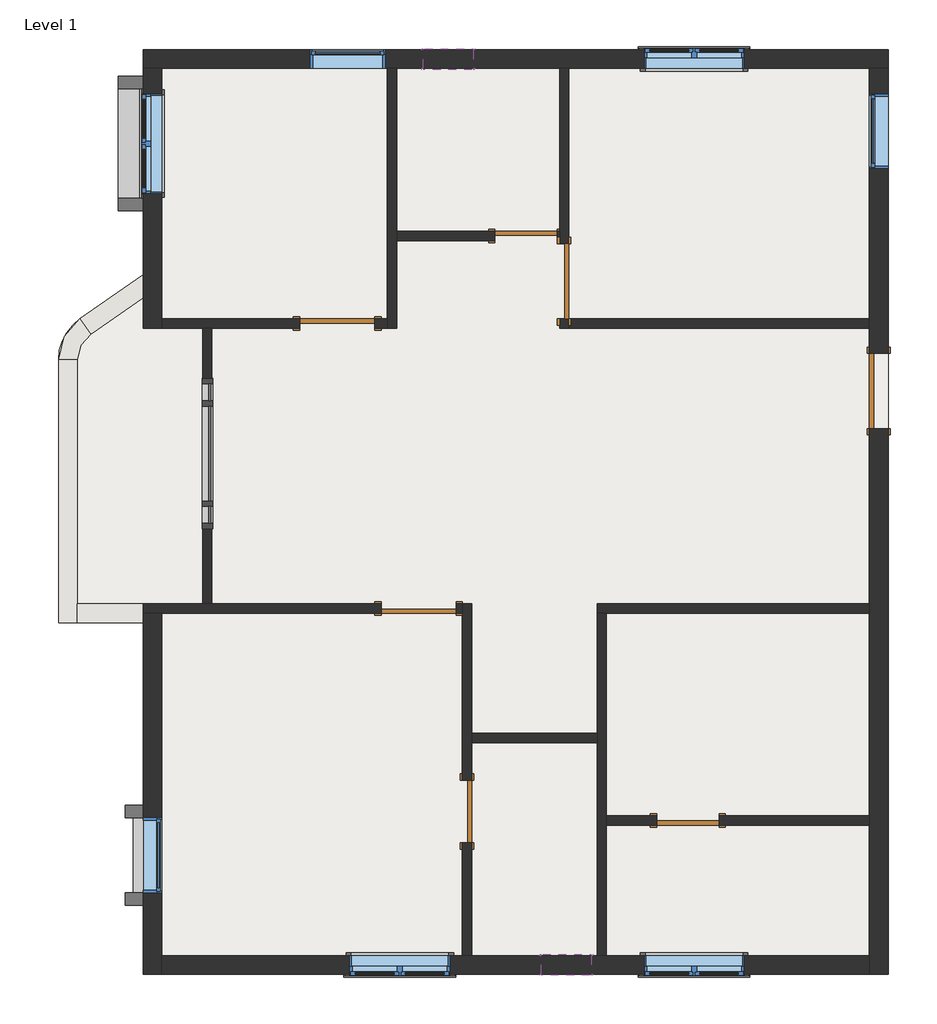
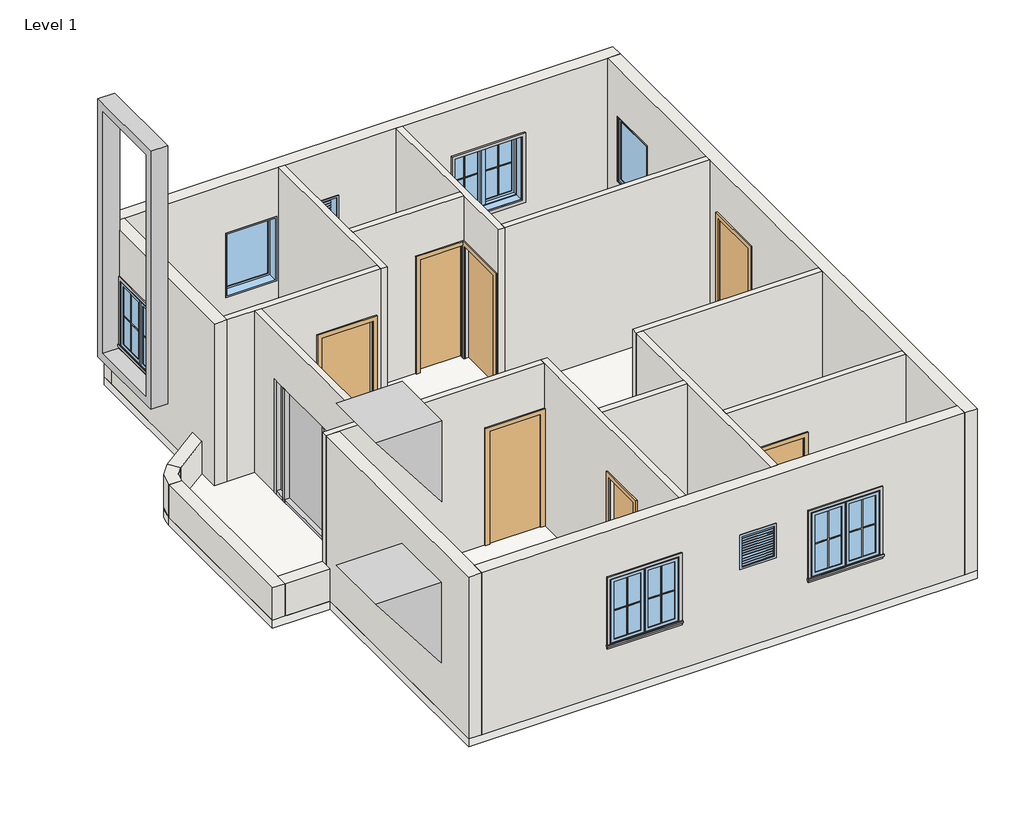
# One storey: 21 walls, 18 proxies, 9 windows, 7 doors, 7 members, 3 plates, 1 slab.
"""IFC4 building model written with IfcOpenShell, lengths in millimetres."""

from ifc_helpers import new_model, si_unit, point, frame, frame_2d, origin, origin_with_axes, place, context, project, spatial, polyline, circle_curve, trimmed, segment, composite_curve, outline, extrude, faceted_brep, transform, mapped, element, save
from components import generic_models_1_generic_models_1_7359c5b6, generic_models_2_generic_models_1_7ae53c19, muntin_pattern_2x2_muntin_pattern_2x2_4dfeb3f3, muntin_pattern_2x2_muntin_pattern_2x2_e852a7e4, trim_window_exterior_flat_with_sill_7cfdd449, trim_window_interior_flat_picture_frame_f1e0b15b, door_214872d5, door_78caadf7, door_e5f9f3c4, door_305aa2a5, door_0ca8825f, member_420b45ef, member_d7472725, member_7cbddb58, member_3374d9b6, system_panel_glazed_b82c55cd, system_panel_glazed_76d7ee11, window_c1f32544, window_af3140d2, window_f2d8fef0

model = new_model("IFC4")

# Units and contexts
model_context = context("Model", 3, world=origin())
ifc_project = project(units=[si_unit("LENGTHUNIT", "METRE", prefix="MILLI")], contexts=[model_context])

# Site, building, storey
site = spatial("IfcSite", under=ifc_project)
building = spatial("IfcBuilding", under=site)
storey = spatial("IfcBuildingStorey", under=building, Name="Level 1", Elevation=0.0)

# Proxies
placement = place(None, origin())
generic_models_1_generic_models_1_shape = generic_models_1_generic_models_1_7359c5b6(model_context)
element("IfcBuildingElementProxy", 1, Name="Generic Models 1 : Generic Models 1", ObjectType="Generic Models 1 : Generic Models 1", at=placement, inside=storey, context=model_context, shape_type="MappedRepresentation", body=[
    mapped(generic_models_1_generic_models_1_shape, transform((0.0, 0.0, 0.0), x_axis=(1.0, 0.0, 0.0), y_axis=(0.0, 1.0, 0.0), z_axis=(0.0, 0.0, 1.0))),
])
generic_models_2_generic_models_1_shape = generic_models_2_generic_models_1_7ae53c19(model_context)
element("IfcBuildingElementProxy", 2, Name="Generic Models 2 : Generic Models 1", ObjectType="Generic Models 2 : Generic Models 1", at=placement, inside=storey, context=model_context, shape_type="MappedRepresentation", body=[
    mapped(generic_models_2_generic_models_1_shape, transform((0.0, 0.0, 0.0), x_axis=(1.0, 0.0, 0.0), y_axis=(0.0, 1.0, 0.0), z_axis=(0.0, 0.0, 1.0))),
])
muntin_pattern_2x2_muntin_pattern_2x2_shape = muntin_pattern_2x2_muntin_pattern_2x2_4dfeb3f3(model_context)
element("IfcBuildingElementProxy", 3, Name="Muntin Pattern_2x2 : Muntin Pattern_2x2", ObjectType="Muntin Pattern_2x2 : Muntin Pattern_2x2", at=placement, inside=storey, context=model_context, shape_type="MappedRepresentation", body=[
    mapped(muntin_pattern_2x2_muntin_pattern_2x2_shape, transform((-15529.7981107, 3990.1340181, 984.25), x_axis=(0.0, 1.0, 0.0), y_axis=(-1.0, 0.0, 0.0), z_axis=(0.0, 0.0, 1.0))),
])
element("IfcBuildingElementProxy", 4, Name="Muntin Pattern_2x2 : Muntin Pattern_2x2", ObjectType="Muntin Pattern_2x2 : Muntin Pattern_2x2", at=placement, inside=storey, context=model_context, shape_type="MappedRepresentation", body=[
    mapped(muntin_pattern_2x2_muntin_pattern_2x2_shape, transform((-9136.9356107, 5426.8215181, 984.25), x_axis=(1.0, 0.0, 0.0), y_axis=(0.0, 1.0, 0.0), z_axis=(0.0, 0.0, 1.0))),
])
element("IfcBuildingElementProxy", 5, Name="Muntin Pattern_2x2 : Muntin Pattern_2x2", ObjectType="Muntin Pattern_2x2 : Muntin Pattern_2x2", at=placement, inside=storey, context=model_context, shape_type="MappedRepresentation", body=[
    mapped(muntin_pattern_2x2_muntin_pattern_2x2_shape, transform((-12111.9106107, -5806.3284819, 984.25), x_axis=(-1.0, 0.0, 0.0), y_axis=(0.0, -1.0, 0.0), z_axis=(0.0, 0.0, 1.0))),
])
element("IfcBuildingElementProxy", 6, Name="Muntin Pattern_2x2 : Muntin Pattern_2x2", ObjectType="Muntin Pattern_2x2 : Muntin Pattern_2x2", at=placement, inside=storey, context=model_context, shape_type="MappedRepresentation", body=[
    mapped(muntin_pattern_2x2_muntin_pattern_2x2_shape, transform((-8530.5106107, -5806.3284819, 984.25), x_axis=(-1.0, 0.0, 0.0), y_axis=(0.0, -1.0, 0.0), z_axis=(0.0, 0.0, 1.0))),
])
muntin_pattern_2x2_muntin_pattern_2x2_2_shape = muntin_pattern_2x2_muntin_pattern_2x2_e852a7e4(model_context)
element("IfcBuildingElementProxy", 7, Name="Muntin Pattern_2x2 : Muntin Pattern_2x2", ObjectType="Muntin Pattern_2x2 : Muntin Pattern_2x2", at=placement, inside=storey, context=model_context, shape_type="MappedRepresentation", body=[
    mapped(muntin_pattern_2x2_muntin_pattern_2x2_2_shape, transform((-15529.7981107, 4596.5590181, 984.25), x_axis=(0.0, -1.0, 0.0), y_axis=(1.0, 0.0, 0.0), z_axis=(0.0, 0.0, 1.0))),
])
element("IfcBuildingElementProxy", 8, Name="Muntin Pattern_2x2 : Muntin Pattern_2x2", ObjectType="Muntin Pattern_2x2 : Muntin Pattern_2x2", at=placement, inside=storey, context=model_context, shape_type="MappedRepresentation", body=[
    mapped(muntin_pattern_2x2_muntin_pattern_2x2_2_shape, transform((-8530.5106107, 5426.8215181, 984.25), x_axis=(-1.0, 0.0, 0.0), y_axis=(0.0, -1.0, 0.0), z_axis=(0.0, 0.0, 1.0))),
])
element("IfcBuildingElementProxy", 9, Name="Muntin Pattern_2x2 : Muntin Pattern_2x2", ObjectType="Muntin Pattern_2x2 : Muntin Pattern_2x2", at=placement, inside=storey, context=model_context, shape_type="MappedRepresentation", body=[
    mapped(muntin_pattern_2x2_muntin_pattern_2x2_2_shape, transform((-12718.3356107, -5806.3284819, 984.25), x_axis=(1.0, 0.0, 0.0), y_axis=(0.0, 1.0, 0.0), z_axis=(0.0, 0.0, 1.0))),
])
element("IfcBuildingElementProxy", 10, Name="Muntin Pattern_2x2 : Muntin Pattern_2x2", ObjectType="Muntin Pattern_2x2 : Muntin Pattern_2x2", at=placement, inside=storey, context=model_context, shape_type="MappedRepresentation", body=[
    mapped(muntin_pattern_2x2_muntin_pattern_2x2_2_shape, transform((-9136.9356107, -5806.3284819, 984.25), x_axis=(1.0, 0.0, 0.0), y_axis=(0.0, 1.0, 0.0), z_axis=(0.0, 0.0, 1.0))),
])
trim_window_exterior_flat_with_sill_shape = trim_window_exterior_flat_with_sill_7cfdd449(model_context)
element("IfcBuildingElementProxy", 11, Name="Trim-Window-Exterior-Flat : with Sill", ObjectType="Trim-Window-Exterior-Flat : with Sill", at=placement, inside=storey, context=model_context, shape_type="MappedRepresentation", body=[
    mapped(trim_window_exterior_flat_with_sill_shape, transform((-15539.3231107, 4293.3465181, 2133.6), x_axis=(0.0, -1.0, 0.0), y_axis=(0.0, 0.0, 1.0), z_axis=(-1.0, 0.0, 0.0))),
])
element("IfcBuildingElementProxy", 12, Name="Trim-Window-Exterior-Flat : with Sill", ObjectType="Trim-Window-Exterior-Flat : with Sill", at=placement, inside=storey, context=model_context, shape_type="MappedRepresentation", body=[
    mapped(trim_window_exterior_flat_with_sill_shape, transform((-8833.7231107, 5436.3465181, 2133.6), x_axis=(-1.0, 0.0, 0.0), y_axis=(0.0, 0.0, 1.0), z_axis=(0.0, 1.0, 0.0))),
])
element("IfcBuildingElementProxy", 13, Name="Trim-Window-Exterior-Flat : with Sill", ObjectType="Trim-Window-Exterior-Flat : with Sill", at=placement, inside=storey, context=model_context, shape_type="MappedRepresentation", body=[
    mapped(trim_window_exterior_flat_with_sill_shape, transform((-12415.1231107, -5815.8534819, 2133.6), x_axis=(1.0, 0.0, 0.0), y_axis=(0.0, 0.0, 1.0), z_axis=(0.0, -1.0, 0.0))),
])
element("IfcBuildingElementProxy", 14, Name="Trim-Window-Exterior-Flat : with Sill", ObjectType="Trim-Window-Exterior-Flat : with Sill", at=placement, inside=storey, context=model_context, shape_type="MappedRepresentation", body=[
    mapped(trim_window_exterior_flat_with_sill_shape, transform((-8833.7231107, -5815.8534819, 2133.6), x_axis=(1.0, 0.0, 0.0), y_axis=(0.0, 0.0, 1.0), z_axis=(0.0, -1.0, 0.0))),
])
trim_window_interior_flat_picture_frame_shape = trim_window_interior_flat_picture_frame_f1e0b15b(model_context)
element("IfcBuildingElementProxy", 15, Name="Trim-Window-Interior-Flat : Picture Frame", ObjectType="Trim-Window-Interior-Flat : Picture Frame", at=placement, inside=storey, context=model_context, shape_type="MappedRepresentation", body=[
    mapped(trim_window_interior_flat_picture_frame_shape, transform((-15310.7231107, 4293.3465181, 2133.6), x_axis=(0.0, 1.0, 0.0), y_axis=(0.0, 0.0, 1.0), z_axis=(1.0, 0.0, 0.0))),
])
element("IfcBuildingElementProxy", 16, Name="Trim-Window-Interior-Flat : Picture Frame", ObjectType="Trim-Window-Interior-Flat : Picture Frame", at=placement, inside=storey, context=model_context, shape_type="MappedRepresentation", body=[
    mapped(trim_window_interior_flat_picture_frame_shape, transform((-8833.7231107, 5207.7465181, 2133.6), x_axis=(1.0, 0.0, 0.0), y_axis=(0.0, 0.0, 1.0), z_axis=(0.0, -1.0, 0.0))),
])
element("IfcBuildingElementProxy", 17, Name="Trim-Window-Interior-Flat : Picture Frame", ObjectType="Trim-Window-Interior-Flat : Picture Frame", at=placement, inside=storey, context=model_context, shape_type="MappedRepresentation", body=[
    mapped(trim_window_interior_flat_picture_frame_shape, transform((-12415.1231107, -5587.2534819, 2133.6), x_axis=(-1.0, 0.0, 0.0), y_axis=(0.0, 0.0, 1.0), z_axis=(0.0, 1.0, 0.0))),
])
element("IfcBuildingElementProxy", 18, Name="Trim-Window-Interior-Flat : Picture Frame", ObjectType="Trim-Window-Interior-Flat : Picture Frame", at=placement, inside=storey, context=model_context, shape_type="MappedRepresentation", body=[
    mapped(trim_window_interior_flat_picture_frame_shape, transform((-8833.7231107, -5587.2534819, 2133.6), x_axis=(-1.0, 0.0, 0.0), y_axis=(0.0, 0.0, 1.0), z_axis=(0.0, 1.0, 0.0))),
])

# Doors
door_shape = door_214872d5(model_context)
element("IfcDoor", 19, ObjectType="Single-Flush : 2'6\" X 7'", at=placement, inside=storey, context=model_context, shape_type="MappedRepresentation", body=[
    mapped(door_shape, transform((-10878.4231107, 3169.3965181, 0.0), x_axis=(1.0, 0.0, 0.0), y_axis=(0.0, 1.0, 0.0), z_axis=(0.0, 0.0, 1.0))),
])
element("IfcDoor", 20, ObjectType="Single-Flush : 2'6\" X 7'", at=placement, inside=storey, context=model_context, shape_type="MappedRepresentation", body=[
    mapped(door_shape, transform((-8909.9231107, -3942.6034819, 0.0), x_axis=(-1.0, 0.0, 0.0), y_axis=(0.0, -1.0, 0.0), z_axis=(0.0, 0.0, 1.0))),
])
door_2_shape = door_78caadf7(model_context)
element("IfcDoor", 21, ObjectType="Single-Flush : 2'6\" X 7'", at=placement, inside=storey, context=model_context, shape_type="MappedRepresentation", body=[
    mapped(door_2_shape, transform((-11595.9731107, -3834.6534819, 0.0), x_axis=(0.0, 1.0, 0.0), y_axis=(-1.0, 0.0, 0.0), z_axis=(0.0, 0.0, 1.0))),
])
door_3_shape = door_e5f9f3c4(model_context)
element("IfcDoor", 22, ObjectType="Single-Flush : 36\" x 84\"", at=placement, inside=storey, context=model_context, shape_type="MappedRepresentation", body=[
    mapped(door_3_shape, transform((-13177.1231107, 2102.5965181, 0.0), x_axis=(1.0, 0.0, 0.0), y_axis=(0.0, 1.0, 0.0), z_axis=(0.0, 0.0, 1.0))),
])
element("IfcDoor", 23, ObjectType="Single-Flush : 36\" x 84\"", at=placement, inside=storey, context=model_context, shape_type="MappedRepresentation", body=[
    mapped(door_3_shape, transform((-10414.8731107, 2618.6439204, 0.0), x_axis=(0.0, -1.0, 0.0), y_axis=(1.0, 0.0, 0.0), z_axis=(0.0, 0.0, 1.0))),
])
door_4_shape = door_305aa2a5(model_context)
element("IfcDoor", 24, ObjectType="Single-Flush : 36\" x 84\"", at=placement, inside=storey, context=model_context, shape_type="MappedRepresentation", body=[
    mapped(door_4_shape, transform((-12186.5231107, -1364.5034819, 0.0), x_axis=(1.0, 0.0, 0.0), y_axis=(0.0, 1.0, 0.0), z_axis=(0.0, 0.0, 1.0))),
])
door_5_shape = door_0ca8825f(model_context)
element("IfcDoor", 25, ObjectType="Single-Flush : 36\" x 84\"", at=placement, inside=storey, context=model_context, shape_type="MappedRepresentation", body=[
    mapped(door_5_shape, transform((-6585.8231107, 1283.4465181, 0.0), x_axis=(0.0, 1.0, 0.0), y_axis=(-1.0, 0.0, 0.0), z_axis=(0.0, 0.0, 1.0))),
])

# Members
member_shape = member_420b45ef(model_context)
element("IfcMember", 26, ObjectType="Rectangular Mullion : 2.5\" x 5\" rectangular", at=placement, inside=storey, context=model_context, shape_type="MappedRepresentation", body=[
    mapped(member_shape, transform((-14758.2731107, 1372.3465181, 0.0), x_axis=(0.0, 0.0, -1.0), y_axis=(-1.0, 0.0, 0.0), z_axis=(0.0, 1.0, 0.0))),
])
element("IfcMember", 27, ObjectType="Rectangular Mullion : 2.5\" x 5\" rectangular", at=placement, inside=storey, context=model_context, shape_type="MappedRepresentation", body=[
    mapped(member_shape, transform((-14758.2731107, -119.9034819, 0.0), x_axis=(0.0, 0.0, -1.0), y_axis=(-1.0, 0.0, 0.0), z_axis=(0.0, 1.0, 0.0))),
])
member_2_shape = member_d7472725(model_context)
element("IfcMember", 28, ObjectType="Rectangular Mullion : 2.5\" x 5\" rectangular", at=placement, inside=storey, context=model_context, shape_type="MappedRepresentation", body=[
    mapped(member_2_shape, transform((-14758.2731107, 1099.2965181, 0.0), x_axis=(0.0, 0.0, -1.0), y_axis=(-1.0, 0.0, 0.0), z_axis=(0.0, 1.0, 0.0))),
])
member_3_shape = member_7cbddb58(model_context)
element("IfcMember", 29, ObjectType="Rectangular Mullion : 2.5\" x 5\" rectangular", at=placement, inside=storey, context=model_context, shape_type="MappedRepresentation", body=[
    mapped(member_3_shape, transform((-14758.2731107, 1131.0465181, 0.0), x_axis=(0.0, -1.0, 0.0), y_axis=(-1.0, 0.0, 0.0), z_axis=(0.0, 0.0, -1.0))),
])
element("IfcMember", 30, ObjectType="Rectangular Mullion : 2.5\" x 5\" rectangular", at=placement, inside=storey, context=model_context, shape_type="MappedRepresentation", body=[
    mapped(member_3_shape, transform((-14758.2731107, -88.1534819, 0.0), x_axis=(0.0, -1.0, 0.0), y_axis=(-1.0, 0.0, 0.0), z_axis=(0.0, 0.0, -1.0))),
])
member_4_shape = member_3374d9b6(model_context)
element("IfcMember", 31, ObjectType="Rectangular Mullion : 2.5\" x 5\" rectangular", at=placement, inside=storey, context=model_context, shape_type="MappedRepresentation", body=[
    mapped(member_4_shape, transform((-14758.2731107, 1435.8465181, 2133.6), x_axis=(0.0, 1.0, 0.0), y_axis=(-1.0, 0.0, 0.0), z_axis=(0.0, 0.0, 1.0))),
])
element("IfcMember", 32, ObjectType="Rectangular Mullion : 2.5\" x 5\" rectangular", at=placement, inside=storey, context=model_context, shape_type="MappedRepresentation", body=[
    mapped(member_4_shape, transform((-14758.2731107, -392.9534819, 0.0), x_axis=(0.0, -1.0, 0.0), y_axis=(-1.0, 0.0, 0.0), z_axis=(0.0, 0.0, -1.0))),
])

# Plates
system_panel_glazed_shape = system_panel_glazed_b82c55cd(model_context)
element("IfcPlate", 33, ObjectType="System Panel : Glazed", at=placement, inside=storey, context=model_context, shape_type="MappedRepresentation", body=[
    mapped(system_panel_glazed_shape, transform((-14758.2731107, 1267.5715181, 63.5), x_axis=(0.0, -1.0, 0.0), y_axis=(1.0, 0.0, 0.0), z_axis=(0.0, 0.0, 1.0))),
])
element("IfcPlate", 34, ObjectType="System Panel : Glazed", at=placement, inside=storey, context=model_context, shape_type="MappedRepresentation", body=[
    mapped(system_panel_glazed_shape, transform((-14758.2731107, -224.6784819, 63.5), x_axis=(0.0, -1.0, 0.0), y_axis=(1.0, 0.0, 0.0), z_axis=(0.0, 0.0, 1.0))),
])
system_panel_glazed_2_shape = system_panel_glazed_76d7ee11(model_context)
element("IfcPlate", 35, ObjectType="System Panel : Glazed", at=placement, inside=storey, context=model_context, shape_type="MappedRepresentation", body=[
    mapped(system_panel_glazed_2_shape, transform((-14758.2731107, 521.4465181, 63.5), x_axis=(0.0, -1.0, 0.0), y_axis=(1.0, 0.0, 0.0), z_axis=(0.0, 0.0, 1.0))),
])

# Slab
element("IfcSlab", 36, ObjectType="6\"", at=placement, inside=storey, context=model_context, shape_type="SweptSolid", body=[
    extrude(outline(composite_curve([segment(polyline([(-6471.5231107, 5436.3465181), (-6471.5231107, -5815.8534819), (-15539.3231107, -5815.8534819), (-15539.3231107, -1535.9534819), (-16568.0231107, -1535.9534819), (-16568.0231107, 1661.5585867)]), True, "CONTINUOUS"), segment(trimmed(circle_curve(frame_2d((-15958.4231107, 1661.5585867)), 609.6), [point((-16568.0231107, 1661.5585867))], [point((-16308.0753063, 2160.9136729))], False, "CARTESIAN"), True, "CONTINUOUS"), segment(polyline([(-16308.0753063, 2160.9136729), (-15539.3231107, 2699.1997553), (-15539.3231107, 5436.3465181), (-6471.5231107, 5436.3465181)]), True, "CONTINUOUS")], self_intersect=False)), frame((0.0, 0.0, -152.4), z_axis=(0.0, 0.0, 1.0), x_axis=(1.0, 0.0, 0.0)), (0.0, 0.0, 1.0), 152.4),
])

# Walls
element("IfcWall", 37, ObjectType="4.5\"", at=placement, inside=storey, context=model_context, shape_type="Brep", body=[
    faceted_brep([(-12567.5231107, 5207.7465181, 0.0), (-12567.5231107, 2159.7465181, 0.0), (-12567.5231107, 2045.4465181, 0.0), (-12567.5231107, 2045.4465181, 3048.0), (-12567.5231107, 2159.7465181, 3048.0), (-12567.5231107, 5207.7465181, 3048.0), (-12453.2231107, 5207.7465181, 0.0), (-12453.2231107, 5207.7465181, 3048.0), (-12453.2231107, 3226.5465181, 3048.0), (-12453.2231107, 3112.2465181, 3048.0), (-12453.2231107, 2045.4465181, 3048.0), (-12453.2231107, 2045.4465181, 0.0), (-12453.2231107, 3112.2465181, 0.0), (-12453.2231107, 3226.5465181, 0.0)], [[[0, 1, 2, 3, 4, 5]], [[6, 7, 8, 9, 10, 11, 12, 13]], [[2, 1, 0, 6, 13, 12, 11]], [[5, 4, 3, 10, 9, 8, 7]], [[0, 5, 7, 6]], [[3, 2, 11, 10]]]),
])
element("IfcWall", 38, ObjectType="4.5\"", at=placement, inside=storey, context=model_context, shape_type="Brep", body=[
    faceted_brep([(-12719.9231107, 2045.4465181, 2133.6), (-12719.9231107, 2045.4465181, 0.0), (-12567.5231107, 2045.4465181, 0.0), (-12567.5231107, 2045.4465181, 3048.0), (-14701.1231107, 2045.4465181, 3048.0), (-14815.4231107, 2045.4465181, 3048.0), (-15310.7231107, 2045.4465181, 3048.0), (-15310.7231107, 2045.4465181, 0.0), (-14815.4231107, 2045.4465181, 0.0), (-14701.1231107, 2045.4465181, 0.0), (-13634.3231107, 2045.4465181, 0.0), (-13634.3231107, 2045.4465181, 2133.6), (-12567.5231107, 2159.7465181, 0.0), (-12719.9231107, 2159.7465181, 0.0), (-12719.9231107, 2159.7465181, 2133.6), (-13634.3231107, 2159.7465181, 2133.6), (-13634.3231107, 2159.7465181, 0.0), (-15310.7231107, 2159.7465181, 0.0), (-15310.7231107, 2159.7465181, 3048.0), (-12567.5231107, 2159.7465181, 3048.0)], [[[0, 1, 2, 3, 4, 5, 6, 7, 8, 9, 10, 11]], [[12, 13, 14, 15, 16, 17, 18, 19]], [[2, 1, 13, 12]], [[10, 9, 8, 7, 17, 16]], [[6, 5, 4, 3, 19, 18]], [[3, 2, 12, 19]], [[7, 6, 18, 17]], [[14, 13, 1, 0]], [[15, 14, 0, 11]], [[16, 15, 11, 10]]]),
])
element("IfcWall", 39, ObjectType="4.5\"", at=placement, inside=storey, context=model_context, shape_type="Brep", body=[
    faceted_brep([(-10472.0231107, 2161.4439204, 2133.6), (-10472.0231107, 2161.4439204, 0.0), (-10472.0231107, 2045.4465181, 0.0), (-10472.0231107, 2045.4465181, 3048.0), (-10472.0231107, 3112.2465181, 3048.0), (-10472.0231107, 3226.5465181, 3048.0), (-10472.0231107, 5207.7465181, 3048.0), (-10472.0231107, 5207.7465181, 0.0), (-10472.0231107, 3226.5465181, 0.0), (-10472.0231107, 3112.2465181, 0.0), (-10472.0231107, 3075.8439204, 0.0), (-10472.0231107, 3075.8439204, 2133.6), (-10357.7231107, 2045.4465181, 0.0), (-10357.7231107, 2159.7465181, 0.0), (-10357.7231107, 2161.4439204, 0.0), (-10357.7231107, 2161.4439204, 2133.6), (-10357.7231107, 3075.8439204, 2133.6), (-10357.7231107, 3075.8439204, 0.0), (-10357.7231107, 5207.7465181, 0.0), (-10357.7231107, 5207.7465181, 3048.0), (-10357.7231107, 2159.7465181, 3048.0), (-10357.7231107, 2045.4465181, 3048.0)], [[[0, 1, 2, 3, 4, 5, 6, 7, 8, 9, 10, 11]], [[12, 13, 14, 15, 16, 17, 18, 19, 20, 21]], [[2, 1, 14, 13, 12]], [[10, 9, 8, 7, 18, 17]], [[6, 5, 4, 3, 21, 20, 19]], [[7, 6, 19, 18]], [[3, 2, 12, 21]], [[15, 14, 1, 0]], [[16, 15, 0, 11]], [[17, 16, 11, 10]]]),
])
element("IfcWall", 40, ObjectType="4.5\"", at=placement, inside=storey, context=model_context, shape_type="SweptSolid", body=[
    extrude(outline(polyline([(2133.6, -10497.4231107), (0.0, -10497.4231107), (0.0, -10472.0231107), (3048.0, -10472.0231107), (3048.0, -12453.2231107), (0.0, -12453.2231107), (0.0, -11259.4231107), (2133.6, -11259.4231107), (2133.6, -10497.4231107)])), frame((0.0, 3112.2465181, 0.0), z_axis=(0.0, 1.0, 0.0), x_axis=(0.0, 0.0, 1.0)), (0.0, 0.0, 1.0), 114.3),
])
element("IfcWall", 41, ObjectType="4.5\"", at=placement, inside=storey, context=model_context, shape_type="SweptSolid", body=[
    extrude(outline(polyline([(-10357.7231107, 2159.7465181), (-6700.1231107, 2159.7465181), (-6700.1231107, 2045.4465181), (-10357.7231107, 2045.4465181), (-10357.7231107, 2159.7465181)])), origin_with_axes(), (0.0, 0.0, 1.0), 3048.0),
])
element("IfcWall", 42, ObjectType="4.5\"", at=placement, inside=storey, context=model_context, shape_type="Brep", body=[
    faceted_brep([(-6700.1231107, -1307.3534819, 0.0), (-10014.8231107, -1307.3534819, 0.0), (-10014.8231107, -1307.3534819, 3048.0), (-6700.1231107, -1307.3534819, 3048.0), (-6700.1231107, -1421.6534819, 0.0), (-6700.1231107, -1421.6534819, 3048.0), (-9900.5231107, -1421.6534819, 3048.0), (-10014.8231107, -1421.6534819, 3048.0), (-10014.8231107, -1421.6534819, 0.0), (-9900.5231107, -1421.6534819, 0.0)], [[[0, 1, 2, 3]], [[4, 5, 6, 7, 8, 9]], [[1, 0, 4, 9, 8]], [[3, 2, 7, 6, 5]], [[0, 3, 5, 4]], [[2, 1, 8, 7]]]),
])
element("IfcWall", 43, ObjectType="4.5\"", at=placement, inside=storey, context=model_context, shape_type="SweptSolid", body=[
    extrude(outline(polyline([(0.0, -9900.5231107), (0.0, -9290.9231107), (2133.6, -9290.9231107), (2133.6, -8528.9231107), (0.0, -8528.9231107), (0.0, -6700.1231107), (3048.0, -6700.1231107), (3048.0, -9900.5231107), (0.0, -9900.5231107)])), frame((0.0, -3999.7534819, 0.0), z_axis=(0.0, 1.0, 0.0), x_axis=(0.0, 0.0, 1.0)), (0.0, 0.0, 1.0), 114.3),
])
element("IfcWall", 44, ObjectType="4.5\"", at=placement, inside=storey, context=model_context, shape_type="Brep", body=[
    faceted_brep([(-9900.5231107, -5587.2534819, 0.0), (-9900.5231107, -3999.7534819, 0.0), (-9900.5231107, -3885.4534819, 0.0), (-9900.5231107, -1421.6534819, 0.0), (-9900.5231107, -1421.6534819, 3048.0), (-9900.5231107, -3885.4534819, 3048.0), (-9900.5231107, -3999.7534819, 3048.0), (-9900.5231107, -5587.2534819, 3048.0), (-10014.8231107, -5587.2534819, 0.0), (-10014.8231107, -5587.2534819, 3048.0), (-10014.8231107, -2996.4534819, 3048.0), (-10014.8231107, -2882.1534819, 3048.0), (-10014.8231107, -1421.6534819, 3048.0), (-10014.8231107, -1421.6534819, 0.0), (-10014.8231107, -2882.1534819, 0.0), (-10014.8231107, -2996.4534819, 0.0)], [[[0, 1, 2, 3, 4, 5, 6, 7]], [[8, 9, 10, 11, 12, 13, 14, 15]], [[3, 2, 1, 0, 8, 15, 14, 13]], [[7, 6, 5, 4, 12, 11, 10, 9]], [[0, 7, 9, 8]], [[4, 3, 13, 12]]]),
])
element("IfcWall", 45, ObjectType="4.5\"", at=placement, inside=storey, context=model_context, shape_type="Brep", body=[
    faceted_brep([(-11538.8231107, -3453.6534819, 2133.6), (-11538.8231107, -3453.6534819, 0.0), (-11538.8231107, -2996.4534819, 0.0), (-11538.8231107, -2882.1534819, 0.0), (-11538.8231107, -1307.3534819, 0.0), (-11538.8231107, -1307.3534819, 3048.0), (-11538.8231107, -2882.1534819, 3048.0), (-11538.8231107, -2996.4534819, 3048.0), (-11538.8231107, -5587.2534819, 3048.0), (-11538.8231107, -5587.2534819, 0.0), (-11538.8231107, -4215.6534819, 0.0), (-11538.8231107, -4215.6534819, 2133.6), (-11653.1231107, -1307.3534819, 0.0), (-11653.1231107, -1421.6534819, 0.0), (-11653.1231107, -3453.6534819, 0.0), (-11653.1231107, -3453.6534819, 2133.6), (-11653.1231107, -4215.6534819, 2133.6), (-11653.1231107, -4215.6534819, 0.0), (-11653.1231107, -5587.2534819, 0.0), (-11653.1231107, -5587.2534819, 3048.0), (-11653.1231107, -1421.6534819, 3048.0), (-11653.1231107, -1307.3534819, 3048.0)], [[[0, 1, 2, 3, 4, 5, 6, 7, 8, 9, 10, 11]], [[12, 13, 14, 15, 16, 17, 18, 19, 20, 21]], [[10, 9, 18, 17]], [[4, 3, 2, 1, 14, 13, 12]], [[8, 7, 6, 5, 21, 20, 19]], [[9, 8, 19, 18]], [[5, 4, 12, 21]], [[15, 14, 1, 0]], [[16, 15, 0, 11]], [[17, 16, 11, 10]]]),
])
element("IfcWall", 46, ObjectType="4.5\"", at=placement, inside=storey, context=model_context, shape_type="SweptSolid", body=[
    extrude(outline(polyline([(-10014.8231107, -2996.4534819), (-11538.8231107, -2996.4534819), (-11538.8231107, -2882.1534819), (-10014.8231107, -2882.1534819), (-10014.8231107, -2996.4534819)])), origin_with_axes(), (0.0, 0.0, 1.0), 3048.0),
])
element("IfcWall", 47, ObjectType="4.5\"", at=placement, inside=storey, context=model_context, shape_type="Brep", body=[
    faceted_brep([(-11653.1231107, -1307.3534819, 0.0), (-11729.3231107, -1307.3534819, 0.0), (-11729.3231107, -1307.3534819, 2133.6), (-12643.7231107, -1307.3534819, 2133.6), (-12643.7231107, -1307.3534819, 0.0), (-14701.1231107, -1307.3534819, 0.0), (-14815.4231107, -1307.3534819, 0.0), (-15539.3231107, -1307.3534819, 0.0), (-15539.3231107, -1307.3534819, 609.6), (-15539.3231107, -1307.3534819, 3048.0), (-14815.4231107, -1307.3534819, 3048.0), (-14701.1231107, -1307.3534819, 3048.0), (-11653.1231107, -1307.3534819, 3048.0), (-11729.3231107, -1421.6534819, 2133.6), (-11729.3231107, -1421.6534819, 0.0), (-11653.1231107, -1421.6534819, 0.0), (-11653.1231107, -1421.6534819, 3048.0), (-15310.7231107, -1421.6534819, 3048.0), (-15539.3231107, -1421.6534819, 3048.0), (-15539.3231107, -1421.6534819, 0.0), (-15310.7231107, -1421.6534819, 0.0), (-12643.7231107, -1421.6534819, 0.0), (-12643.7231107, -1421.6534819, 2133.6)], [[[0, 1, 2, 3, 4, 5, 6, 7, 8, 9, 10, 11, 12]], [[13, 14, 15, 16, 17, 18, 19, 20, 21, 22]], [[15, 14, 1, 0]], [[21, 20, 19, 7, 6, 5, 4]], [[12, 11, 10, 9, 18, 17, 16]], [[0, 12, 16, 15]], [[2, 1, 14, 13]], [[3, 2, 13, 22]], [[4, 3, 22, 21]], [[7, 19, 18, 9, 8]]]),
])
element("IfcWall", 48, ObjectType="4.5\"", at=placement, inside=storey, context=model_context, shape_type="SweptSolid", body=[
    extrude(outline(polyline([(-1307.3534819, 3048.0), (2045.4465181, 3048.0), (2045.4465181, 0.0), (1435.8465181, 0.0), (1435.8465181, 2133.6), (-392.9534819, 2133.6), (-392.9534819, 0.0), (-1307.3534819, 0.0), (-1307.3534819, 3048.0)])), frame((-14815.4231107, 0.0, 0.0), z_axis=(1.0, 0.0, 0.0), x_axis=(0.0, 1.0, 0.0)), (0.0, 0.0, 1.0), 114.3),
])
element("IfcWall", 49, ObjectType="9\"", at=placement, inside=storey, context=model_context, shape_type="Brep", body=[
    faceted_brep([(-15539.3231107, 5207.7465181, 0.0), (-15310.7231107, 5207.7465181, 0.0), (-12567.5231107, 5207.7465181, 0.0), (-12453.2231107, 5207.7465181, 0.0), (-10472.0231107, 5207.7465181, 0.0), (-10357.7231107, 5207.7465181, 0.0), (-6700.1231107, 5207.7465181, 0.0), (-6471.5231107, 5207.7465181, 0.0), (-6471.5231107, 5207.7465181, 3048.0), (-6700.1231107, 5207.7465181, 3048.0), (-10357.7231107, 5207.7465181, 3048.0), (-10472.0231107, 5207.7465181, 3048.0), (-12453.2231107, 5207.7465181, 3048.0), (-12567.5231107, 5207.7465181, 3048.0), (-15310.7231107, 5207.7465181, 3048.0), (-15539.3231107, 5207.7465181, 3048.0), (-12129.3731107, 5207.7465181, 2133.6), (-11519.7731107, 5207.7465181, 2133.6), (-11519.7731107, 5207.7465181, 1524.0), (-12129.3731107, 5207.7465181, 1524.0), (-8224.1231107, 5207.7465181, 2133.6), (-8224.1231107, 5207.7465181, 914.4), (-9443.3231107, 5207.7465181, 914.4), (-9443.3231107, 5207.7465181, 2133.6), (-12592.9231107, 5207.7465181, 2133.6), (-12592.9231107, 5207.7465181, 914.4), (-13507.3231107, 5207.7465181, 914.4), (-13507.3231107, 5207.7465181, 2133.6), (-15539.3231107, 5436.3465181, 0.0), (-15539.3231107, 5436.3465181, 3048.0), (-6471.5231107, 5436.3465181, 3048.0), (-6471.5231107, 5436.3465181, 0.0), (-12129.3731107, 5436.3465181, 2133.6), (-12129.3731107, 5436.3465181, 1524.0), (-11519.7731107, 5436.3465181, 1524.0), (-11519.7731107, 5436.3465181, 2133.6), (-8224.1231107, 5436.3465181, 2133.6), (-9443.3231107, 5436.3465181, 2133.6), (-9443.3231107, 5436.3465181, 914.4), (-8224.1231107, 5436.3465181, 914.4), (-12592.9231107, 5436.3465181, 2133.6), (-13507.3231107, 5436.3465181, 2133.6), (-13507.3231107, 5436.3465181, 914.4), (-12592.9231107, 5436.3465181, 914.4)], [[[0, 1, 2, 3, 4, 5, 6, 7, 8, 9, 10, 11, 12, 13, 14, 15], [16, 17, 18, 19], [20, 21, 22, 23], [24, 25, 26, 27]], [[28, 29, 30, 31], [32, 33, 34, 35], [36, 37, 38, 39], [40, 41, 42, 43]], [[7, 6, 5, 4, 3, 2, 1, 0, 28, 31]], [[15, 14, 13, 12, 11, 10, 9, 8, 30, 29]], [[0, 15, 29, 28]], [[8, 7, 31, 30]], [[33, 32, 16, 19]], [[34, 33, 19, 18]], [[35, 34, 18, 17]], [[32, 35, 17, 16]], [[21, 20, 36, 39]], [[22, 21, 39, 38]], [[23, 22, 38, 37]], [[20, 23, 37, 36]], [[25, 24, 40, 43]], [[26, 25, 43, 42]], [[27, 26, 42, 41]], [[24, 27, 41, 40]]]),
])
element("IfcWall", 50, ObjectType="9\"", at=placement, inside=storey, context=model_context, shape_type="Brep", body=[
    faceted_brep([(-15539.3231107, 5207.7465181, 0.0), (-15539.3231107, 2699.1997553, 0.0), (-15539.3231107, 2420.1306843, 0.0), (-15539.3231107, 2045.4465181, 0.0), (-15539.3231107, 2045.4465181, 3048.0), (-15539.3231107, 5207.7465181, 3048.0), (-15539.3231107, 4902.9465181, 2133.6), (-15539.3231107, 3683.7465181, 2133.6), (-15539.3231107, 3683.7465181, 914.4), (-15539.3231107, 4902.9465181, 914.4), (-15310.7231107, 5207.7465181, 0.0), (-15310.7231107, 5207.7465181, 3048.0), (-15310.7231107, 2159.7465181, 3048.0), (-15310.7231107, 2045.4465181, 3048.0), (-15310.7231107, 2045.4465181, 0.0), (-15310.7231107, 2159.7465181, 0.0), (-15310.7231107, 4902.9465181, 2133.6), (-15310.7231107, 4902.9465181, 914.4), (-15310.7231107, 3683.7465181, 914.4), (-15310.7231107, 3683.7465181, 2133.6)], [[[0, 1, 2, 3, 4, 5], [6, 7, 8, 9]], [[10, 11, 12, 13, 14, 15], [16, 17, 18, 19]], [[3, 2, 1, 0, 10, 15, 14]], [[5, 4, 13, 12, 11]], [[0, 5, 11, 10]], [[4, 3, 14, 13]], [[17, 16, 6, 9]], [[18, 17, 9, 8]], [[19, 18, 8, 7]], [[16, 19, 7, 6]]]),
])
element("IfcWall", 51, ObjectType="9\"", at=placement, inside=storey, context=model_context, shape_type="Brep", body=[
    faceted_brep([(-6700.1231107, 5207.7465181, 0.0), (-6700.1231107, 2159.7465181, 0.0), (-6700.1231107, 2045.4465181, 0.0), (-6700.1231107, 1740.6465181, 0.0), (-6700.1231107, 1740.6465181, 2133.6), (-6700.1231107, 826.2465181, 2133.6), (-6700.1231107, 826.2465181, 0.0), (-6700.1231107, -1307.3534819, 0.0), (-6700.1231107, -1421.6534819, 0.0), (-6700.1231107, -3885.4534819, 0.0), (-6700.1231107, -3999.7534819, 0.0), (-6700.1231107, -5587.2534819, 0.0), (-6700.1231107, -5815.8534819, 0.0), (-6700.1231107, -5815.8534819, 3048.0), (-6700.1231107, -5587.2534819, 3048.0), (-6700.1231107, -3999.7534819, 3048.0), (-6700.1231107, -3885.4534819, 3048.0), (-6700.1231107, -1421.6534819, 3048.0), (-6700.1231107, -1307.3534819, 3048.0), (-6700.1231107, 2045.4465181, 3048.0), (-6700.1231107, 2159.7465181, 3048.0), (-6700.1231107, 5207.7465181, 3048.0), (-6700.1231107, 4902.9465181, 2133.6), (-6700.1231107, 3988.5465181, 2133.6), (-6700.1231107, 3988.5465181, 914.4), (-6700.1231107, 4902.9465181, 914.4), (-6471.5231107, 1740.6465181, 2133.6), (-6471.5231107, 1740.6465181, 0.0), (-6471.5231107, 5207.7465181, 0.0), (-6471.5231107, 5207.7465181, 3048.0), (-6471.5231107, -5815.8534819, 3048.0), (-6471.5231107, -5815.8534819, 0.0), (-6471.5231107, 826.2465181, 0.0), (-6471.5231107, 826.2465181, 2133.6), (-6471.5231107, 4902.9465181, 2133.6), (-6471.5231107, 4902.9465181, 914.4), (-6471.5231107, 3988.5465181, 914.4), (-6471.5231107, 3988.5465181, 2133.6)], [[[0, 1, 2, 3, 4, 5, 6, 7, 8, 9, 10, 11, 12, 13, 14, 15, 16, 17, 18, 19, 20, 21], [22, 23, 24, 25]], [[26, 27, 28, 29, 30, 31, 32, 33], [34, 35, 36, 37]], [[32, 31, 12, 11, 10, 9, 8, 7, 6]], [[28, 27, 3, 2, 1, 0]], [[21, 20, 19, 18, 17, 16, 15, 14, 13, 30, 29]], [[0, 21, 29, 28]], [[13, 12, 31, 30]], [[35, 34, 22, 25]], [[36, 35, 25, 24]], [[37, 36, 24, 23]], [[34, 37, 23, 22]], [[4, 3, 27, 26]], [[5, 4, 26, 33]], [[6, 5, 33, 32]]]),
])
element("IfcWall", 52, ObjectType="9\"", at=placement, inside=storey, context=model_context, shape_type="Brep", body=[
    faceted_brep([(-15310.7231107, -5815.8534819, 0.0), (-6700.1231107, -5815.8534819, 0.0), (-6700.1231107, -5815.8534819, 3048.0), (-15310.7231107, -5815.8534819, 3048.0), (-10084.6731107, -5815.8534819, 2133.6), (-10084.6731107, -5815.8534819, 1524.0), (-10694.2731107, -5815.8534819, 1524.0), (-10694.2731107, -5815.8534819, 2133.6), (-13024.7231107, -5815.8534819, 2133.6), (-11805.5231107, -5815.8534819, 2133.6), (-11805.5231107, -5815.8534819, 914.4), (-13024.7231107, -5815.8534819, 914.4), (-9443.3231107, -5815.8534819, 2133.6), (-8224.1231107, -5815.8534819, 2133.6), (-8224.1231107, -5815.8534819, 914.4), (-9443.3231107, -5815.8534819, 914.4), (-15310.7231107, -5587.2534819, 0.0), (-15310.7231107, -5587.2534819, 3048.0), (-11653.1231107, -5587.2534819, 3048.0), (-11538.8231107, -5587.2534819, 3048.0), (-10014.8231107, -5587.2534819, 3048.0), (-9900.5231107, -5587.2534819, 3048.0), (-6700.1231107, -5587.2534819, 3048.0), (-6700.1231107, -5587.2534819, 0.0), (-9900.5231107, -5587.2534819, 0.0), (-10014.8231107, -5587.2534819, 0.0), (-11538.8231107, -5587.2534819, 0.0), (-11653.1231107, -5587.2534819, 0.0), (-10084.6731107, -5587.2534819, 2133.6), (-10694.2731107, -5587.2534819, 2133.6), (-10694.2731107, -5587.2534819, 1524.0), (-10084.6731107, -5587.2534819, 1524.0), (-13024.7231107, -5587.2534819, 2133.6), (-13024.7231107, -5587.2534819, 914.4), (-11805.5231107, -5587.2534819, 914.4), (-11805.5231107, -5587.2534819, 2133.6), (-9443.3231107, -5587.2534819, 2133.6), (-9443.3231107, -5587.2534819, 914.4), (-8224.1231107, -5587.2534819, 914.4), (-8224.1231107, -5587.2534819, 2133.6)], [[[0, 1, 2, 3], [4, 5, 6, 7], [8, 9, 10, 11], [12, 13, 14, 15]], [[16, 17, 18, 19, 20, 21, 22, 23, 24, 25, 26, 27], [28, 29, 30, 31], [32, 33, 34, 35], [36, 37, 38, 39]], [[1, 0, 16, 27, 26, 25, 24, 23]], [[3, 2, 22, 21, 20, 19, 18, 17]], [[0, 3, 17, 16]], [[2, 1, 23, 22]], [[5, 4, 28, 31]], [[6, 5, 31, 30]], [[7, 6, 30, 29]], [[4, 7, 29, 28]], [[33, 32, 8, 11]], [[34, 33, 11, 10]], [[35, 34, 10, 9]], [[32, 35, 9, 8]], [[37, 36, 12, 15]], [[38, 37, 15, 14]], [[39, 38, 14, 13]], [[36, 39, 13, 12]]]),
])
element("IfcWall", 53, ObjectType="9\"", at=placement, inside=storey, context=model_context, shape_type="Brep", body=[
    faceted_brep([(-15539.3231107, -1421.6534819, 3048.0), (-15539.3231107, -1421.6534819, 0.0), (-15539.3231107, -1535.9534819, 0.0), (-15539.3231107, -5815.8534819, 0.0), (-15539.3231107, -5815.8534819, 3048.0), (-15539.3231107, -4825.2534819, 2133.6), (-15539.3231107, -4825.2534819, 914.4), (-15539.3231107, -3910.8534819, 914.4), (-15539.3231107, -3910.8534819, 2133.6), (-15310.7231107, -1421.6534819, 0.0), (-15310.7231107, -1421.6534819, 3048.0), (-15310.7231107, -5587.2534819, 3048.0), (-15310.7231107, -5815.8534819, 3048.0), (-15310.7231107, -5815.8534819, 0.0), (-15310.7231107, -5587.2534819, 0.0), (-15310.7231107, -4825.2534819, 2133.6), (-15310.7231107, -3910.8534819, 2133.6), (-15310.7231107, -3910.8534819, 914.4), (-15310.7231107, -4825.2534819, 914.4)], [[[0, 1, 2, 3, 4], [5, 6, 7, 8]], [[9, 10, 11, 12, 13, 14], [15, 16, 17, 18]], [[3, 2, 1, 9, 14, 13]], [[0, 4, 12, 11, 10]], [[4, 3, 13, 12]], [[0, 10, 9, 1]], [[6, 5, 15, 18]], [[7, 6, 18, 17]], [[8, 7, 17, 16]], [[5, 8, 16, 15]]]),
])
element("IfcWall", 54, ObjectType="9\"", at=placement, inside=storey, context=model_context, shape_type="Brep", body=[
    faceted_brep([(-16339.4231107, -1535.9534819, 0.0), (-16339.4231107, -1307.3534819, 0.0), (-16339.4231107, 1661.5585867, 0.0), (-16339.4231107, 1661.5585867, 609.6), (-16339.4231107, -1307.3534819, 609.6), (-16339.4231107, -1535.9534819, 609.6), (-16568.0231107, -1535.9534819, 0.0), (-16568.0231107, -1535.9534819, 609.6), (-16568.0231107, 1661.5585867, 609.6), (-16568.0231107, 1661.5585867, 0.0)], [[[0, 1, 2, 3, 4, 5]], [[6, 7, 8, 9]], [[2, 1, 0, 6, 9]], [[3, 2, 9, 8]], [[5, 4, 3, 8, 7]], [[0, 5, 7, 6]]]),
])
element("IfcWall", 55, ObjectType="9\"", at=placement, inside=storey, context=model_context, shape_type="Brep", body=[
    faceted_brep([(-15539.3231107, -1307.3534819, 0.0), (-16339.4231107, -1307.3534819, 0.0), (-16339.4231107, -1307.3534819, 609.6), (-15539.3231107, -1307.3534819, 609.6), (-15539.3231107, -1535.9534819, 0.0), (-15539.3231107, -1535.9534819, 609.6), (-16339.4231107, -1535.9534819, 609.6), (-16339.4231107, -1535.9534819, 0.0), (-15539.3231107, -1421.6534819, 0.0)], [[[0, 1, 2, 3]], [[4, 5, 6, 7]], [[1, 0, 8, 4, 7]], [[3, 2, 6, 5]], [[0, 3, 5, 4, 8]], [[2, 1, 7, 6]]]),
])
element("IfcWall", 56, ObjectType="9\"", at=placement, inside=storey, context=model_context, shape_type="SweptSolid", body=[
    extrude(outline(polyline([(-15539.3231107, 2420.1306843), (-16176.9557329, 1973.6555156), (-16308.0753063, 2160.9136729), (-15539.3231107, 2699.1997553), (-15539.3231107, 2420.1306843)])), origin_with_axes(), (0.0, 0.0, 1.0), 609.6),
])
element("IfcWall", 57, ObjectType="9\"", at=placement, inside=storey, context=model_context, shape_type="SweptSolid", body=[
    extrude(outline(composite_curve([segment(polyline([(-16308.0753063, 2160.9136729), (-16176.9557329, 1973.6555156)]), True, "CONTINUOUS"), segment(trimmed(circle_curve(frame_2d((-15958.4231107, 1661.5585867)), 381.0), [point((-16176.9557329, 1973.6555156))], [point((-16339.4231107, 1661.5585867))], True, "CARTESIAN"), True, "CONTINUOUS"), segment(polyline([(-16339.4231107, 1661.5585867), (-16568.0231107, 1661.5585867)]), True, "CONTINUOUS"), segment(trimmed(circle_curve(frame_2d((-15958.4231107, 1661.5585867)), 609.6), [point((-16568.0231107, 1661.5585867))], [point((-16308.0753063, 2160.9136729))], False, "CARTESIAN"), True, "CONTINUOUS")], self_intersect=False)), origin_with_axes(), (0.0, 0.0, 1.0), 609.6),
])

# Windows
window_shape = window_c1f32544(model_context)
element("IfcWindow", 58, ObjectType="Fixed : 36\" x 48\"", at=placement, inside=storey, context=model_context, shape_type="MappedRepresentation", body=[
    mapped(window_shape, transform((-13012.0231107, 5322.0465181, 0.0), x_axis=(1.0, 0.0, 0.0), y_axis=(0.0, 1.0, 0.0), z_axis=(0.0, 0.0, 1.0))),
])
element("IfcWindow", 59, ObjectType="Fixed : 36\" x 48\"", at=placement, inside=storey, context=model_context, shape_type="MappedRepresentation", body=[
    mapped(window_shape, transform((-6585.8231107, 4483.8465181, 0.0), x_axis=(0.0, 1.0, 0.0), y_axis=(-1.0, 0.0, 0.0), z_axis=(0.0, 0.0, 1.0))),
])
element("IfcWindow", 60, ObjectType="Fixed : 36\" x 48\"", at=placement, inside=storey, context=model_context, shape_type="MappedRepresentation", body=[
    mapped(window_shape, transform((-15425.0231107, -4406.1534819, 0.0), x_axis=(0.0, -1.0, 0.0), y_axis=(1.0, 0.0, 0.0), z_axis=(0.0, 0.0, 1.0))),
])
window_2_shape = window_af3140d2(model_context)
element("IfcWindow", 61, ObjectType="Window-Casement-Double : 48\" x 48\"", at=placement, inside=storey, context=model_context, shape_type="MappedRepresentation", body=[
    mapped(window_2_shape, transform((-15425.0231107, 4293.3465181, 0.0), x_axis=(0.0, 1.0, 0.0), y_axis=(-1.0, 0.0, 0.0), z_axis=(0.0, 0.0, 1.0))),
])
element("IfcWindow", 62, ObjectType="Window-Casement-Double : 48\" x 48\"", at=placement, inside=storey, context=model_context, shape_type="MappedRepresentation", body=[
    mapped(window_2_shape, transform((-8833.7231107, 5322.0465181, 0.0), x_axis=(1.0, 0.0, 0.0), y_axis=(0.0, 1.0, 0.0), z_axis=(0.0, 0.0, 1.0))),
])
element("IfcWindow", 63, ObjectType="Window-Casement-Double : 48\" x 48\"", at=placement, inside=storey, context=model_context, shape_type="MappedRepresentation", body=[
    mapped(window_2_shape, transform((-12415.1231107, -5701.5534819, 0.0), x_axis=(-1.0, 0.0, 0.0), y_axis=(0.0, -1.0, 0.0), z_axis=(0.0, 0.0, 1.0))),
])
element("IfcWindow", 64, ObjectType="Window-Casement-Double : 48\" x 48\"", at=placement, inside=storey, context=model_context, shape_type="MappedRepresentation", body=[
    mapped(window_2_shape, transform((-8833.7231107, -5701.5534819, 0.0), x_axis=(-1.0, 0.0, 0.0), y_axis=(0.0, -1.0, 0.0), z_axis=(0.0, 0.0, 1.0))),
])
window_3_shape = window_f2d8fef0(model_context)
element("IfcWindow", 65, ObjectType="Window-Louvers : 24\" x 24\"", at=placement, inside=storey, context=model_context, shape_type="MappedRepresentation", body=[
    mapped(window_3_shape, transform((-11824.5731107, 5328.3965181, 609.6), x_axis=(1.0, 0.0, 0.0), y_axis=(0.0, 1.0, 0.0), z_axis=(0.0, 0.0, 1.0))),
])
element("IfcWindow", 66, ObjectType="Window-Louvers : 24\" x 24\"", at=placement, inside=storey, context=model_context, shape_type="MappedRepresentation", body=[
    mapped(window_3_shape, transform((-10389.4731107, -5707.9034819, 609.6), x_axis=(-1.0, 0.0, 0.0), y_axis=(0.0, -1.0, 0.0), z_axis=(0.0, 0.0, 1.0))),
])

save(model, "model.ifc")

# Revit data of these elements
# Type "Muntin Pattern_2x2 : Muntin Pattern_2x2"
#   Width [instance default] = 4' - 0"
#   Thickness = 0' - 0 1/2"
#   Height [instance default] = 4' - 0"
#   Distance = 0' - 0 3/4"
#   Interior Material [instance default] = none
#   Exterior Material [instance default] = none
#   Default Elevation = 0
# Type "Trim-Window-Exterior-Flat : with Sill"
#   Trim Width = 0' - 2 1/4"
#   Trim Thickness_Picture Frame = 0' - 1 1/4"
#   Trim Thickness_with Sill = 0' - 0 3/4"
#   Sill Thickness = 0' - 1 1/4"
#   Opening Width [instance default] = 2' - 0"
#   Opening Height [instance default] = 3' - 0"
#   Default Elevation = 4' - 0"
#   Sill = yes
#   Picture Frame = no
#   Trim Material [instance default] = none
# Type "Trim-Window-Interior-Flat : Picture Frame"
#   Trim Thickness_Picture Frame = 0' - 1 1/4"
#   Trim Width = 0' - 2 1/4"
#   Trim Thickness_with Sill = 0' - 0 3/4"
#   Sill Thickness = 0' - 1 1/4"
#   Opening Width [instance default] = 2' - 0"
#   Opening Height [instance default] = 3' - 0"
#   Default Elevation = 4' - 0"
#   Sill = no
#   Picture Frame = yes
#   Trim Material [instance default] = none
# Type "Single-Flush : 2'6\" X 7'"
#   Type Mark = "8"
#   Construction Type Id = "MDOOR"
#   Assembly Code = "C1020"
#   Analytic Construction = "Metal"
#   Thickness = 0' - 2"
#   Heat Transfer Coefficient (U) = 0.651978 BTU/(h·ft²·°F)
#   Height = 7' - 0"
#   Trim Projection Ext = 0' - 1"
#   Trim Projection Int = 0' - 1"
#   Trim Width = 0' - 3"
#   Width = 2' - 6"
#   Define Thermal Properties by = 1
#   Door Material = Door - Panel
#   Frame Material = Door - Frame
#   Visual Light Transmittance = 0
#   Solar Heat Gain Coefficient = 0
#   Function = (empty or 0)
#   Wall Closure = (empty or 0)
# Type "Single-Flush : 36\" x 84\""
#   Type Mark = "1"
#   Construction Type Id = "MDOOR"
#   Assembly Code = "C1020"
#   Analytic Construction = "Metal"
#   Thickness = 0' - 2"
#   Heat Transfer Coefficient (U) = 0.651978 BTU/(h·ft²·°F)
#   Height = 7' - 0"
#   Trim Projection Ext = 0' - 1"
#   Trim Projection Int = 0' - 1"
#   Trim Width = 0' - 3"
#   Width = 3' - 0"
#   Define Thermal Properties by = 1
#   Define Thermal Properties by = 1
#   Door Material = Door - Panel
#   Frame Material = Door - Frame
#   Visual Light Transmittance = 0
#   Solar Heat Gain Coefficient = 0
#   Function = (empty or 0)
#   Wall Closure = (empty or 0)
# Type "Rectangular Mullion : 2.5\" x 5\" rectangular"
#   built-in parameter 1007304 = 0.416667 (stored number, unit not read)
#   built-in parameter 1007301 = 0.104167 (stored number, unit not read)
#   built-in parameter 1007300 = 0.104167 (stored number, unit not read)
# Type "System Panel : Glazed"
#   Construction Type Id = "GSP4R"
#   Analytic Construction = "1/8 in Pilkington single glazing"
#   Visual Light Transmittance = 0.9
#   Solar Heat Gain Coefficient = 0.86
#   Heat Transfer Coefficient (U) = 1.18115 BTU/(h·ft²·°F)
#   Define Thermal Properties by = 1
# Type "6\""
#   Assembly Code = "B1010"
#   Function = 0
#   Layers, outside or top first: 0' - 6" no material (function 1)
# Type "4.5\""
#   Assembly Code = "B2010"
#   Layers, outside or top first: 0' - 4 1/2" no material (function 1)
# Type "9\""
#   Assembly Code = "B2010"
#   Layers, outside or top first: 0' - 9" no material (function 1)
# Type "Fixed : 36\" x 48\""
#   Type Mark = "W2"
#   Construction Type Id = "GSP4R"
#   Assembly Code = "B2020100"
#   Analytic Construction = "1/8 in Pilkington single glazing"
#   Visual Light Transmittance = 0.9
#   Solar Heat Gain Coefficient = 0.78
#   Heat Transfer Coefficient (U) = 0.6496 BTU/(h·ft²·°F)
#   Height = 4' - 0"
#   Default Sill Height = 3' - 0"
#   Width = 3' - 0"
#   Window Inset = 0' - 0 3/4"
#   Define Thermal Properties by = 1
#   Define Thermal Properties by = 1
#   Glass Pane Material = Glass
#   Sash Material = Sash
#   Wall Closure = (empty or 0)
# Type "Window-Casement-Double : 48\" x 48\""
#   Type Mark = "W"
#   Fire Rating = "0.5h"
#   Assembly Code = "B2020100"
#   Analytic Construction = "Double glazing - domestic"
#   Frame Extension [instance default] = 0' - 0 1/4"
#   Window Inset [instance default] = 0' - 0"
#   Wall Thickness [instance default] = 0' - 6"
#   Interior Wall Closure [instance default] = 0' - 2 1/4"
#   Half Width = 2' - 0"
#   Visual Light Transmittance = 0.81
#   Thermal Resistance (R) = 1.8146 (h·ft²·°F)/BTU
#   Solar Heat Gain Coefficient = 0.76
#   Rough Width = 4' - 0 1/2"
#   Rough Height = 4' - 0 1/2"
#   Height = 4' - 0"
#   Heat Transfer Coefficient (U) = 0.5511 BTU/(h·ft²·°F)
#   Exterior Wall Closure [instance default] = 0' - 1 1/4"
#   Extension Jamb [instance default] = 0' - 2 1/4"
#   Default Sill Height = 3' - 0"
#   Width = 4' - 0"
#   Define Thermal Properties by = 0
#   Muntin Visibility = yes
#   Interior Trim Visibility [instance default] = yes
#   Exterior Trim Visibility [instance default] = yes
#   Extension Jamb Visibility [instance default] = yes
#   Interior Trim Material = Wood - Stained
#   Muntin Pattern = Muntin Pattern_2x2 : Muntin Pattern_2x2
#   Interior Trim = Trim-Window-Interior-Flat : Picture Frame
#   Interior Frame Material = Wood - Stained
#   Glass Panel Material = Glass
#   Exterior Trim Material = Clad - White
#   Exterior Trim = Trim-Window-Exterior-Flat : with Sill
#   Exterior Frame Material = Clad - White
#   Wall Closure = (empty or 0)
# Type "Window-Louvers : 24\" x 24\""
#   Type Mark = "V"
#   Construction Type Id = "GSP4R"
#   Assembly Code = "B20"
#   Analytic Construction = "1/8 in Pilkington single glazing"
#   Visual Light Transmittance = 0.9
#   Thermal Resistance (R) = 1.53941 (h·ft²·°F)/BTU
#   Solar Heat Gain Coefficient = 0.78
#   Max Height = 1' - 11.74264"
#   Height = 2' - 0"
#   Heat Transfer Coefficient (U) = 0.6496 BTU/(h·ft²·°F)
#   Blade Width [instance default] = 1' - 10 1/2"
#   Blade Vertical Thickness = 0' - 0.35355"
#   Blade Thickness = 0' - 0 1/4"
#   Blade Spacing = 0' - 1 1/2"
#   Blade Height = 0' - 1.85355"
#   Blade Depth = 0' - 3"
#   Blade Angle = 45.00°
#   Default Sill Height = 3' - 0"
#   Trim Projection_Exterior = 0' - 0 1/2"
#   Trim Projection_Interior = 0' - 0 1/2"
#   Trim Width_Exterior = 0' - 1 1/2"
#   Trim Width_Interior = 0' - 1 1/2"
#   Width = 2' - 0"
#   Max Blade Count = 12
#   Define Thermal Properties by = 1
#   Blade Count = 12
#   Frame Material = Birch
#   Louver Material = Birch
#   Trim Exterior Material = Birch
#   Trim Interior Material = Birch
#   Wall Closure = (empty or 0)
# Element 1 (IfcBuildingElementProxy, "Generic Models 1 : Generic Models 1")
#   Phase Created = New Construction
# Element 2 (IfcBuildingElementProxy, "Generic Models 2 : Generic Models 1")
#   Phase Created = New Construction
# Elements 3, 4, 5, 6, 7, 8, 9, 10 (IfcBuildingElementProxy, "Muntin Pattern_2x2 : Muntin Pattern_2x2")
#   Width = 1' - 6 5/8"
#   Height = 3' - 6 1/2"
#   Interior Material = Wood - Stained
#   Exterior Material = Clad - White
#   Phase Created = New Construction
#   Materials on its faces: "Clad - White", "Wood - Stained"
# Elements 11, 12, 13, 14 (IfcBuildingElementProxy, "Trim-Window-Exterior-Flat : with Sill")
#   Opening Width = 4' - 0"
#   Opening Height = 4' - 0"
#   Trim Material = Clad - White
#   Phase Created = New Construction
#   Materials on its faces: "Clad - White"
# Elements 15, 16, 17, 18 (IfcBuildingElementProxy, "Trim-Window-Interior-Flat : Picture Frame")
#   Opening Width = 4' - 0"
#   Opening Height = 4' - 0"
#   Trim Material = Wood - Stained
#   Phase Created = New Construction
#   Materials on its faces: "Wood - Stained"
# Elements 19, 20, 21 (IfcDoor, "Single-Flush : 2'6\" X 7'")
#   Phase Created = New Construction
#   Materials on its faces: "Door - Frame", "Door - Panel"
# Elements 22, 23, 24, 25 (IfcDoor, "Single-Flush : 36\" x 84\"")
#   Phase Created = New Construction
#   Materials on its faces: "Door - Frame", "Door - Panel"
# Elements 26, 27, 28, 29, 30, 31, 32 (IfcMember, "Rectangular Mullion : 2.5\" x 5\" rectangular")
#   Phase Created = New Construction
#   Materials on its faces: "Aluminum"
# Elements 33, 34, 35 (IfcPlate, "System Panel : Glazed")
#   Phase Created = New Construction
#   Materials on its faces: "Glass"
# Element 36 (IfcSlab, "6\"")
#   Height Offset From Level = 0' - 0"
#   Phase Created = New Construction
#   Materials on its faces: "Default Floor"
# Elements 37, 38, 39, 40, 41, 42, 43, 44, 45, 46, 47, 48 (IfcWall, "4.5\"")
#   Top Offset = 0' - 0"
#   Base Offset = 0' - 0"
#   wall height = 10' - 0"
#   Phase Created = New Construction
#   Base Constraint = Level 1
#   Top Constraint = Level 2
#   Materials on its faces: "Default Wall"
# Elements 49, 50, 51, 52, 53 (IfcWall, "9\"")
#   Top Offset = 0' - 0"
#   Base Offset = 0' - 0"
#   wall height = 10' - 0"
#   Phase Created = New Construction
#   Base Constraint = Level 1
#   Top Constraint = Level 2
#   Materials on its faces: "Default Wall"
# Elements 54, 55, 56 (IfcWall, "9\"")
#   Top Offset = -8' - 0"
#   Base Offset = 0' - 0"
#   wall height = 2' - 0"
#   Phase Created = New Construction
#   Base Constraint = Level 1
#   Top Constraint = Level 2
#   Materials on its faces: "Default Wall"
# Element 57 (IfcWall, "9\"")
#   Top Offset = -8' - 0"
#   Base Offset = 0' - 0"
#   Unconnected Height = 20' - 0"
#   wall height = 2' - 0"
#   Phase Created = New Construction
#   Materials on its faces: "Default Wall"
# Element 58 (IfcWindow, "Fixed : 36\" x 48\"")
#   Mark = "8"
#   Phase Created = New Construction
#   Materials on its faces: "Sash", "Glass"
# Element 59 (IfcWindow, "Fixed : 36\" x 48\"")
#   Mark = "9"
#   Phase Created = New Construction
#   Materials on its faces: "Sash", "Glass"
# Element 60 (IfcWindow, "Fixed : 36\" x 48\"")
#   Mark = "10"
#   Phase Created = New Construction
#   Materials on its faces: "Sash", "Glass"
# Element 61 (IfcWindow, "Window-Casement-Double : 48\" x 48\"")
#   Mark = "4"
#   Window Inset = 0' - 0"
#   Interior Wall Closure = 0' - 2 1/4"
#   Frame Extension = 0' - 0 1/4"
#   Exterior Wall Closure = 0' - 1 1/4"
#   Interior Trim Visibility = yes
#   Exterior Trim Visibility = yes
#   Phase Created = New Construction
#   Materials on its faces: "Wood - Stained", "Glass", "Clad - White"
# Element 62 (IfcWindow, "Window-Casement-Double : 48\" x 48\"")
#   Mark = "5"
#   Window Inset = 0' - 0"
#   Interior Wall Closure = 0' - 2 1/4"
#   Frame Extension = 0' - 0 1/4"
#   Exterior Wall Closure = 0' - 1 1/4"
#   Interior Trim Visibility = yes
#   Exterior Trim Visibility = yes
#   Phase Created = New Construction
#   Materials on its faces: "Wood - Stained", "Glass", "Clad - White"
# Element 63 (IfcWindow, "Window-Casement-Double : 48\" x 48\"")
#   Mark = "6"
#   Window Inset = 0' - 0"
#   Interior Wall Closure = 0' - 2 1/4"
#   Frame Extension = 0' - 0 1/4"
#   Exterior Wall Closure = 0' - 1 1/4"
#   Interior Trim Visibility = yes
#   Exterior Trim Visibility = yes
#   Phase Created = New Construction
#   Materials on its faces: "Wood - Stained", "Glass", "Clad - White"
# Element 64 (IfcWindow, "Window-Casement-Double : 48\" x 48\"")
#   Mark = "7"
#   Window Inset = 0' - 0"
#   Interior Wall Closure = 0' - 2 1/4"
#   Frame Extension = 0' - 0 1/4"
#   Exterior Wall Closure = 0' - 1 1/4"
#   Interior Trim Visibility = yes
#   Exterior Trim Visibility = yes
#   Phase Created = New Construction
#   Materials on its faces: "Wood - Stained", "Glass", "Clad - White"
# Element 65 (IfcWindow, "Window-Louvers : 24\" x 24\"")
#   Mark = "1"
#   Blade Width = 1' - 10 1/2"
#   Phase Created = New Construction
#   Materials on its faces: "Birch"
# Element 66 (IfcWindow, "Window-Louvers : 24\" x 24\"")
#   Mark = "2"
#   Blade Width = 1' - 10 1/2"
#   Phase Created = New Construction
#   Materials on its faces: "Birch"
# Materials
#   "Door - Panel": class "Wood", colour RGB 210 159 95, transparency 0, Cost = 0
#   "Door - Frame": colour RGB 118 70 51, transparency 0, Cost = 0
#   "Glass": class "Glass", colour RGB 0 128 192, transparency 0.75, Description = "Soda Lime Glass", Cost = 0
#   "Sash": class "Wood", colour RGB 224 178 126, transparency 0, Cost = 0
#   "Wood - Stained": class "Wood", colour RGB 224 178 126, transparency 0, Cost = 0
#   "Clad - White": class "Wood", colour RGB 242 242 238, transparency 0, Cost = 0
#   "Birch": class "Wood", colour RGB 224 178 126, transparency 0, Description = "Betula Alleghaniensis", Cost = 0
#   "Aluminum": class "Metal", colour RGB 247 247 247, transparency 0, Description = "Aluminum 6061", Cost = 0
